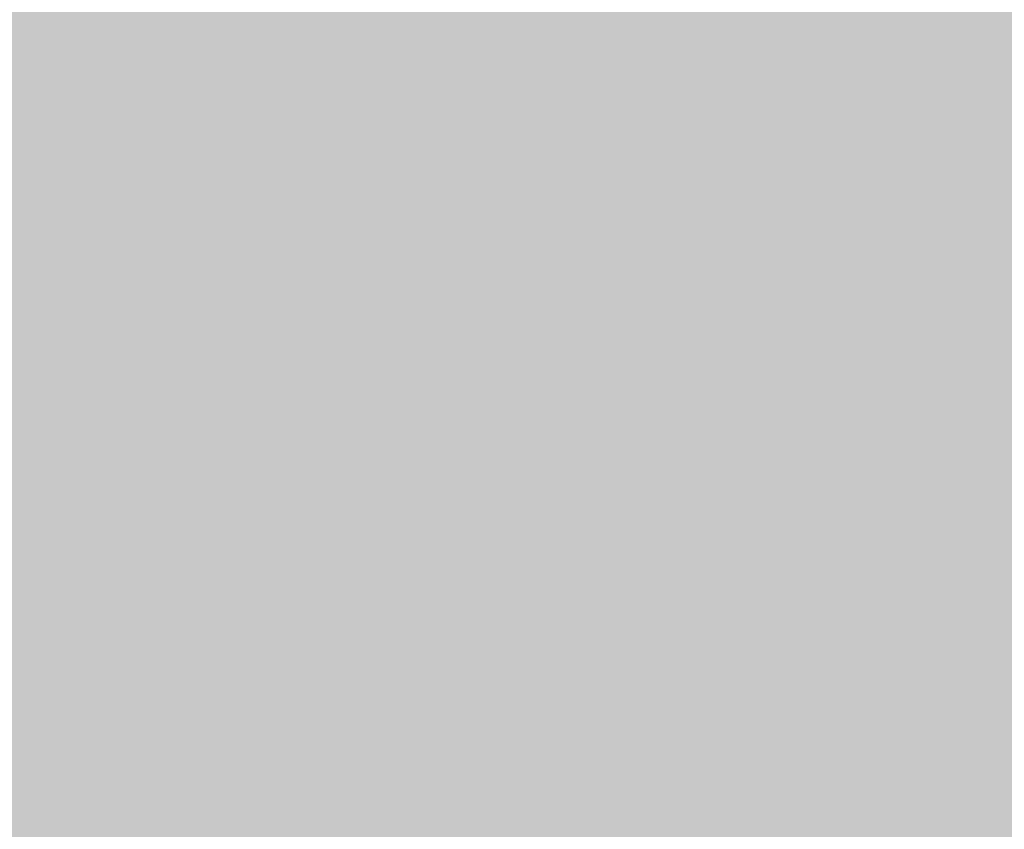
# Model space of a CAD drawing. Units: feet. Extents: x 3168 to 4724, y 827 to 1477.
# Tile 214 of 256: x 3363.87 to 3379.08, y 1074.89 to 1087.4. Entities that reach past the tile are written whole.
import ezdxf

# ---------------------------------------------------------------- set-up
doc = ezdxf.new("R2010")
doc.units = ezdxf.units.FT
doc.layers.add('A-ELEV-PATT', color=8, linetype='Continuous', lineweight=13)

msp = doc.modelspace()

# ---------------------------------------------------------------- hatches: boundary and pattern name
at = {"layer": 'A-ELEV-PATT'}
h = msp.add_hatch(color=256, dxfattribs=at)
h.dxf.hatch_style = 1
edge = h.paths.add_edge_path()
edge.add_ellipse((3552.906, 979.22), major_axis=(36.745, 0), ratio=0.484848, start_angle=0, end_angle=360)
edge = h.paths.add_edge_path()
edge.add_ellipse((3559.892, 929.252), major_axis=(36.745, 0), ratio=0.484848, start_angle=0, end_angle=360)
edge = h.paths.add_edge_path()
edge.add_line((3299.317, 1198.606), (3479.917, 1198.606))
edge.add_line((3479.917, 1198.606), (3479.917, 1209.869))
edge.add_spline(control_points=[(3479.917, 1209.869), (3464.301, 1209.869), (3448.686, 1209.869), (3410.949, 1209.869), (3388.828, 1209.869), (3355.647, 1209.869), (3344.586, 1209.869), (3327.996, 1209.869), (3322.466, 1209.869), (3314.17, 1209.869), (3311.405, 1209.869), (3307.257, 1209.869), (3305.875, 1209.869), (3303.801, 1209.869), (3303.11, 1209.869), (3302.073, 1209.869), (3301.727, 1209.869), (3301.209, 1209.869), (3301.036, 1209.869), (3300.777, 1209.869), (3300.69, 1209.869), (3300.561, 1209.869), (3300.517, 1209.869), (3300.453, 1209.869), (3300.431, 1209.869), (3300.399, 1209.869), (3300.388, 1209.869), (3300.366, 1209.869), (3300.346, 1209.869), (3300.346, 1209.869), (3300.346, 1209.869), (3300.343, 1209.869), (3300.341, 1209.869), (3300.338, 1209.869), (3300.337, 1209.869), (3300.334, 1209.869), (3300.332, 1209.869), (3300.326, 1209.869), (3300.321, 1209.869), (3300.311, 1209.869), (3300.306, 1209.869), (3300.291, 1209.869), (3300.28, 1209.869), (3300.232, 1209.869), (3300.195, 1209.869), (3299.951, 1209.871), (3299.745, 1209.874), (3299.437, 1209.883), (3299.334, 1209.887), (3299.181, 1209.893), (3299.13, 1209.895), (3298.652, 1209.917), (3298.229, 1209.946), (3297.602, 1210.002), (3297.393, 1210.023), (3297.083, 1210.058), (3296.979, 1210.07), (3296.293, 1210.155), (3295.718, 1210.243), (3294.869, 1210.399), (3294.588, 1210.454), (3294.169, 1210.543), (3294.03, 1210.574), (3291.707, 1211.101), (3289.654, 1211.813), (3285.776, 1213.564), (3283.951, 1214.603), (3280.512, 1216.98), (3278.897, 1218.318), (3276.38, 1220.829), (3275.416, 1221.918), (3274.039, 1223.708), (3273.581, 1224.35), (3273.143, 1225.016)], knot_values=[39.119033, 39.119033, 39.119033, 39.119033, 39.286353, 39.286353, 39.523379, 39.523379, 39.641892, 39.641892, 39.701148, 39.701148, 39.730777, 39.730777, 39.745591, 39.745591, 39.752998, 39.752998, 39.756701, 39.756701, 39.758553, 39.758553, 39.759479, 39.759479, 39.759942, 39.759942, 39.760173, 39.760173, 39.760289, 39.760289, 39.760405, 39.760405, 39.760463, 39.760463, 39.763389, 39.763389, 39.764851, 39.764851, 39.767304, 39.767304, 39.773825, 39.773825, 39.78057, 39.78057, 39.79477, 39.79477, 39.845194, 39.845194, 40.126715, 40.126715, 40.267476, 40.267476, 40.337856, 40.337856, 40.927023, 40.927023, 41.221606, 41.221606, 41.368898, 41.368898, 42.202622, 42.202622, 42.619485, 42.619485, 42.827916, 42.827916, 46.118323, 46.118323, 49.408731, 49.408731, 52.699139, 52.699139, 54.927489, 54.927489, 56.104228, 56.104228, 56.104228, 56.104228], weights=[1, 1, 1, 1, 1, 1, 1, 1, 1, 1, 1, 1, 1, 1, 1, 1, 1, 1, 1, 1, 1, 1, 1, 1, 1, 1, 1, 1, 1, 1, 1, 1, 1, 1, 1, 1, 1, 1, 1, 1, 1, 1, 1, 1, 1, 1, 1, 1, 1, 1, 1, 1, 1, 1, 1, 1, 1, 1, 1, 1, 1, 1, 1, 1, 1, 1, 1, 1, 1, 1, 1, 1, 1, 1], degree=3, periodic=0)
edge.add_line((3273.143, 1225.016), (3273.143, 1099.016))
edge.add_line((3273.143, 1099.016), (3299.317, 1099.016))
edge.add_line((3299.317, 1099.016), (3299.317, 1198.606))
edge = h.paths.add_edge_path()
edge.add_line((3304.758, 1324.158), (3479.917, 1324.158))
edge.add_line((3479.917, 1324.158), (3479.917, 1335.715))
edge.add_line((3479.917, 1335.715), (3269.162, 1335.715))
edge.add_spline(control_points=[(3269.162, 1335.715), (3264.024, 1335.715), (3258.364, 1328.958), (3259.264, 1323.9)], knot_values=[0, 0, 0, 0, 15.412191, 15.412191, 15.412191, 15.412191], degree=3, periodic=0)
edge.add_line((3259.264, 1323.9), (3265.517, 1288.769))
edge.add_line((3265.517, 1288.769), (3275.265, 1261.546))
edge.add_line((3275.265, 1261.546), (3304.758, 1261.546))
edge.add_line((3304.758, 1261.546), (3304.758, 1324.158))
h = msp.add_hatch(color=256, dxfattribs=at)
h.dxf.hatch_style = 1
h.paths.add_polyline_path([(3384.525, 1099.016), (3335.029, 1099.016), (3299.317, 1099.016), (3273.143, 1099.016), (3217.565, 1099.016), (3168.069, 827.116), (3335.029, 827.116)])

doc.saveas('drawing.dxf')
